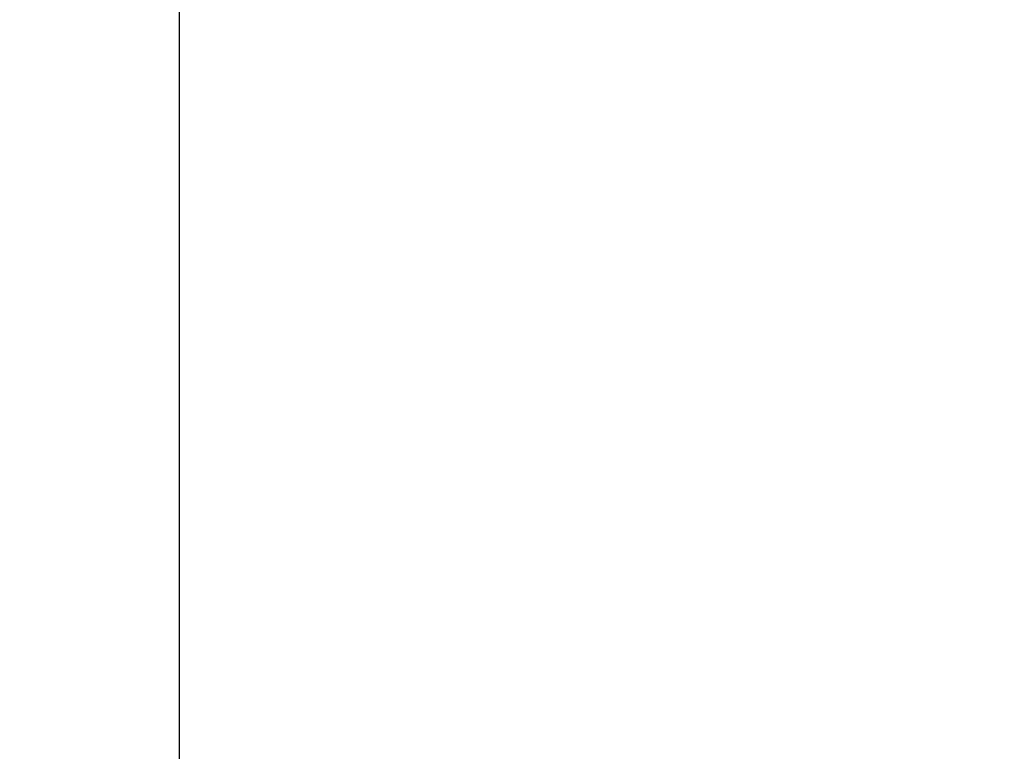
# Model space of a CAD drawing. Units: inches. Extents: x -48 to 50072, y 0 to 21068.
# Tile 13 of 75: x 212 to 236, y 330 to 347. Entities that reach past the tile are written whole.
import ezdxf

# ---------------------------------------------------------------- set-up
doc = ezdxf.new("R2010")
doc.units = ezdxf.units.IN
doc.header["$MEASUREMENT"] = 0
doc.layers.add('A-ANNO-DIMS', color=2, linetype='Continuous', lineweight=18)
doc.styles.get("Standard").update_dxf_attribs({"font": 'arial.ttf'})
doc.dimstyles.get("Standard").update_dxf_attribs({"dimtxt": 8, "dimasz": 0.18, "dimexe": 0.18, "dimexo": 0.0625, "dimgap": 0.09, "dimtad": 0, "dimtih": 1, "dimtoh": 1, "dimdec": 1, "dimzin": 0, "dimdsep": 46, "dimlunit": 4, "dimtxsty": 'Standard', "dimblk": 'ARCHTICK', "dimcen": 0.09, "dimadec": 0, "dimazin": 0, "dimtfac": 1, "dimtdec": 1, "dimtofl": 0, "dimtmove": 0, "dimatfit": 3, "dimldrblk": 'ARCHTICK', "dimfxl": 1, "dimtolj": 1, "dimtzin": 0, "dimarcsym": 0})

# ---------------------------------------------------------------- blocks, each defined once
blk = doc.blocks.new('_ArchTick')
at = {"color": 0, "linetype": 'ByBlock', "const_width": 0.15}
blk.add_lwpolyline([(-0.5, -0.5), (0.5, 0.5)], dxfattribs=at)
blk = doc.blocks.new('*D116')
at = {"layer": 'A-ANNO-DIMS', "color": 0, "lineweight": -2, "transparency": 16777216}
for p, q in [((18.017, 677.712), (18.017, 165.945)), ((216.017, 677.712), (216.017, 165.945)), ((18.017, 166.125), (108.458, 166.125)), ((216.017, 166.125), (125.576, 166.125))]:
    blk.add_line(p, q, dxfattribs=at)
at = {"layer": 'Defpoints', "color": 0, "transparency": 16777216}
for p in [(18.017, 677.775), (216.017, 677.775), (216.017, 166.125)]:
    blk.add_point(p, dxfattribs=at)
at = {"layer": 'A-ANNO-DIMS', "color": 0, "lineweight": -2, "transparency": 16777216, "xscale": 0.18, "yscale": 0.18, "zscale": 0.18, "rotation": 180}
blk.add_blockref('_ArchTick', (18.017, 166.125), dxfattribs=at)
at = {"layer": 'A-ANNO-DIMS', "color": 0, "lineweight": -2, "transparency": 16777216, "xscale": 0.18, "yscale": 0.18, "zscale": 0.18}
blk.add_blockref('_ArchTick', (216.017, 166.125), dxfattribs=at)
at = {"layer": 'A-ANNO-DIMS', "color": 0, "transparency": 16777216, "insert": (117.017, 166.125), "char_height": 8, "attachment_point": 5}
blk.add_mtext('\\A1;198', dxfattribs=at)
blk = doc.blocks.new('*D117')
at = {"layer": 'A-ANNO-DIMS', "color": 0, "lineweight": -2, "transparency": 16777216}
for p, q in [((216.017, 488.712), (216.017, 165.945)), ((297.017, 488.712), (297.017, 165.945)), ((216.017, 166.125), (251.464, 166.125)), ((297.017, 166.125), (261.57, 166.125))]:
    blk.add_line(p, q, dxfattribs=at)
at = {"layer": 'Defpoints', "color": 0, "transparency": 16777216}
for p in [(216.017, 488.775), (297.017, 488.775), (297.017, 166.125)]:
    blk.add_point(p, dxfattribs=at)
at = {"layer": 'A-ANNO-DIMS', "color": 0, "lineweight": -2, "transparency": 16777216, "xscale": 0.18, "yscale": 0.18, "zscale": 0.18, "rotation": 180}
blk.add_blockref('_ArchTick', (216.017, 166.125), dxfattribs=at)
at = {"layer": 'A-ANNO-DIMS', "color": 0, "lineweight": -2, "transparency": 16777216, "xscale": 0.18, "yscale": 0.18, "zscale": 0.18}
blk.add_blockref('_ArchTick', (297.017, 166.125), dxfattribs=at)
at = {"layer": 'A-ANNO-DIMS', "color": 0, "transparency": 16777216, "insert": (256.517, 166.125), "char_height": 8, "attachment_point": 5}
blk.add_mtext('\\A1;81', dxfattribs=at)

msp = doc.modelspace()

# ---------------------------------------------------------------- dimensions: what is measured, and where the dimension line sits
at = {"layer": 'A-ANNO-DIMS'}
for base, p1, p2, picture, middle in [((216.017, 166.125), (18.017, 677.775), (216.017, 677.775), '*D116', (117.017, 166.125)), ((297.017, 166.125), (216.017, 488.775), (297.017, 488.775), '*D117', (256.517, 166.125))]:
    dim = msp.add_linear_dim(base=base, p1=p1, p2=p2, dimstyle='Standard', override={"dimdec": 0, "dimlfac": 1, "dimrnd": 0, "dimzin": 0, "dimdsep": 46, "dimlunit": 2}, dxfattribs=at)
    dim.commit()
    dim.dimension.update_dxf_attribs({"geometry": picture, "text_midpoint": middle})

doc.saveas('drawing.dxf')
